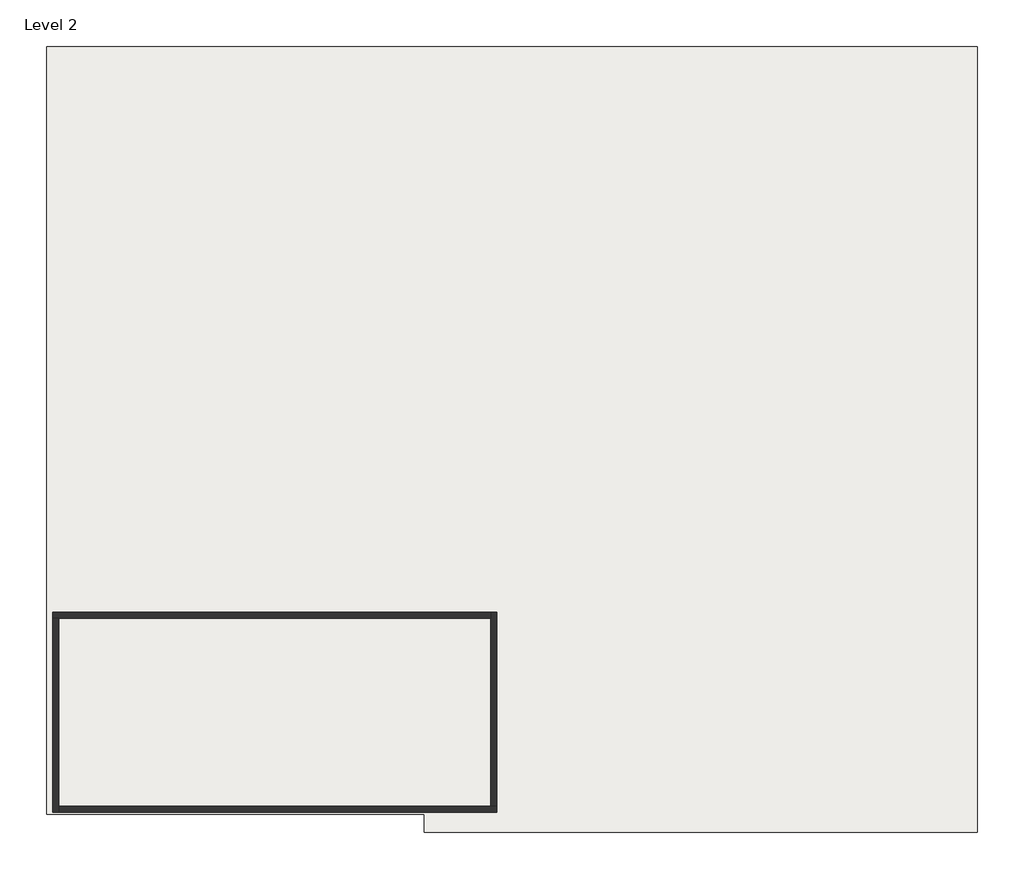
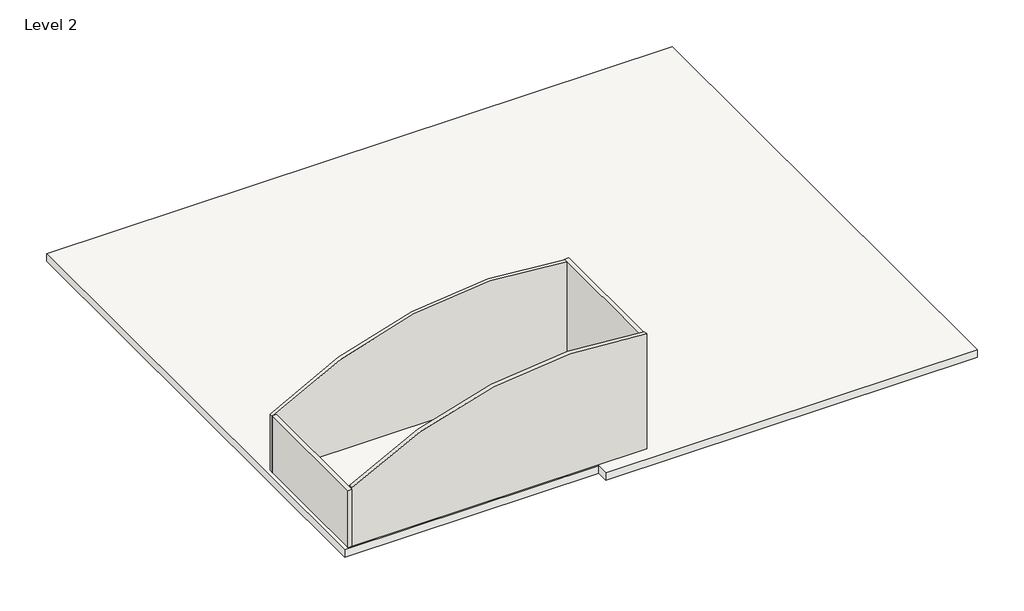
# One storey: 4 walls, 1 slab.
"""IFC4 building model written with IfcOpenShell, lengths in millimetres."""

from ifc_helpers import new_model, si_unit, frame, origin, place, context, project, spatial, polyline, circle_curve, outline, extrude, faceted_brep, element, save
from ifc_brep_helpers import plane_surface, cylinder_surface, advanced_brep

model = new_model("IFC4")

# Units and contexts
model_context = context("Model", 3, world=origin())
ifc_project = project(units=[si_unit("LENGTHUNIT", "METRE", prefix="MILLI")], contexts=[model_context])

# Site, building, storey
site = spatial("IfcSite", under=ifc_project)
building = spatial("IfcBuilding", under=site)
storey = spatial("IfcBuildingStorey", under=building, Name="Level 2", Elevation=5696.0)

# Slab
placement = place(None, origin())
element("IfcSlab", 1, ObjectType="Generic 5\"", at=placement, inside=storey, context=model_context, shape_type="SweptSolid", body=[
    extrude(outline(polyline([(-21609.2828737, 17887.7099289), (9680.512328, 17887.7099289), (9680.512328, -8525.0900711), (-8912.287672, -8525.0900711), (-8912.287672, -7915.4900711), (-21609.2828737, -7915.4900711), (-21609.2828737, 17887.7099289)])), frame((0.0, 0.0, 5296.0), z_axis=(0.0, 0.0, 1.0), x_axis=(1.0, 0.0, 0.0)), (0.0, 0.0, 1.0), 400.0),
])

# Walls
element("IfcWall", 2, ObjectType="Generic - 9\"", at=placement, inside=storey, context=model_context, shape_type="AdvancedBrep", body=[
    advanced_brep(
    [(-6474.0828737, -7653.4043927, 5696.0), (-6674.0828737, -7653.4043927, 5696.0), (-21204.4828737, -7653.4043927, 5696.0), (-21204.4828737, -7653.4043927, 8808.0736123), (-6474.0828737, -7653.4043927, 11775.1398494), (-6474.0828737, -7653.4043927, 11709.4744332), (-6474.0828737, -7853.4043927, 5696.0), (-6474.0828737, -7853.4043927, 11775.1398494), (-21204.4828737, -7853.4043927, 8808.0736123), (-21204.4828737, -7853.4043927, 8723.1502964), (-21204.4828737, -7853.4043927, 5696.0)],
    [
        (0, 1),
        (1, 2),
        (2, 3),
        (3, 4, circle_curve(frame((-9994.1657461, -7653.4043927, -8797.995189), z_axis=(0.0, 1.0, 0.0), x_axis=(1.0, 0.0, 0.0)), 20872.107434)),
        (4, 5),
        (5, 0),
        (6, 7),
        (7, 8, circle_curve(frame((-9994.1657461, -7853.4043927, -8797.995189), z_axis=(0.0, -1.0, 0.0), x_axis=(1.0, 0.0, 0.0)), 20872.107434)),
        (8, 9),
        (9, 10),
        (10, 6),
        (4, 7),
        (6, 0),
        (2, 10),
        (8, 3),
    ],
    [
        plane_surface(frame((-6574.0828737, -7653.4043927, 5696.0), z_axis=(0.0, 1.0, 0.0), x_axis=(-1.0, 0.0, 0.0))),
        plane_surface(frame((-6574.0828737, -7853.4043927, 5696.0), z_axis=(0.0, -1.0, 0.0), x_axis=(1.0, 0.0, 0.0))),
        plane_surface(frame((-6474.0828737, -1657.4043927, 5696.0), z_axis=(1.0, 0.0, 0.0), x_axis=(0.0, 1.0, 0.0))),
        plane_surface(frame((-21204.4828737, -7753.4043927, 5696.0), z_axis=(-1.0, 0.0, 0.0), x_axis=(0.0, 1.0, 0.0))),
        plane_surface(frame((-6574.0828737, -7653.4043927, 5696.0), z_axis=(0.0, 0.0, -1.0), x_axis=(0.0, -1.0, 0.0))),
        cylinder_surface(frame((-9994.1657461, -7853.4043927, -8797.995189), z_axis=(0.0, 1.0, 0.0), x_axis=(1.0, 0.0, 0.0)), 20872.107434),
    ],
    [
        (0, [[1, 2, 3, 4, 5, 6]]),
        (1, [[7, 8, 9, 10, 11]]),
        (2, [[-6, -5, 12, -7, 13]]),
        (3, [[-3, 14, -10, -9, 15]]),
        (4, [[-2, -1, -13, -11, -14]]),
        (5, [[-4, -15, -8, -12]]),
    ],
),
])
element("IfcWall", 3, ObjectType="Generic - 9\"", at=placement, inside=storey, context=model_context, shape_type="Brep", body=[
    faceted_brep([(-6674.0828737, -1123.0109022, 5696.0), (-6674.0828737, -1323.0109022, 5696.0), (-6674.0828737, -7653.4043927, 5696.0), (-6674.0828737, -7653.4043927, 11709.4744332), (-6674.0828737, -1123.0109022, 11709.4744332), (-6674.0828737, -1123.0109022, 11691.648024), (-6474.0828737, -1123.0109022, 5696.0), (-6474.0828737, -1123.0109022, 11709.4744332), (-6474.0828737, -7653.4043927, 11709.4744332), (-6474.0828737, -7653.4043927, 5696.0)], [[[0, 1, 2, 3, 4, 5]], [[6, 7, 8, 9]], [[2, 1, 0, 6, 9]], [[4, 3, 8, 7]], [[3, 2, 9, 8]], [[0, 5, 4, 7, 6]]]),
])
element("IfcWall", 4, ObjectType="Generic - 9\"", at=placement, inside=storey, context=model_context, shape_type="AdvancedBrep", body=[
    advanced_brep(
    [(-21404.4828737, -1323.0109022, 5696.0), (-21204.4828737, -1323.0109022, 5696.0), (-6674.0828737, -1323.0109022, 5696.0), (-6674.0828737, -1323.0109022, 11691.648024), (-21404.4828737, -1323.0109022, 8677.877941), (-21404.4828737, -1123.0109022, 5696.0), (-21404.4828737, -1123.0109022, 8677.877941), (-6674.0828737, -1123.0109022, 11691.648024), (-6674.0828737, -1123.0109022, 5696.0)],
    [
        (0, 1),
        (1, 2),
        (2, 3),
        (3, 4, circle_curve(frame((-10324.9947486, -1323.0109022, -7969.5581139), z_axis=(0.0, -1.0, 0.0), x_axis=(-1.0, 0.0, 0.0)), 19997.3044262)),
        (4, 0),
        (5, 6),
        (6, 7, circle_curve(frame((-10324.9947486, -1123.0109022, -7969.5581139), z_axis=(0.0, 1.0, 0.0), x_axis=(-1.0, 0.0, 0.0)), 19997.3044262)),
        (7, 8),
        (8, 5),
        (2, 8),
        (7, 3),
        (4, 6),
        (5, 0),
    ],
    [
        plane_surface(frame((-21204.4828737, -1323.0109022, 5696.0), z_axis=(0.0, -1.0, 0.0), x_axis=(1.0, 0.0, 0.0))),
        plane_surface(frame((-21204.4828737, -1123.0109022, 5696.0), z_axis=(0.0, 1.0, 0.0), x_axis=(-1.0, 0.0, 0.0))),
        plane_surface(frame((-6674.0828737, -1657.4043927, 5696.0), z_axis=(1.0, 0.0, 0.0), x_axis=(0.0, -1.0, 0.0))),
        plane_surface(frame((-21404.4828737, -7753.4043927, 5696.0), z_axis=(-1.0, 0.0, 0.0), x_axis=(0.0, -1.0, 0.0))),
        plane_surface(frame((-21304.4828737, -1323.0109022, 5696.0), z_axis=(0.0, 0.0, -1.0), x_axis=(0.0, 1.0, 0.0))),
        cylinder_surface(frame((-10324.9947486, -1123.0109022, -7969.5581139), z_axis=(0.0, -1.0, 0.0), x_axis=(-1.0, 0.0, 0.0)), 19997.3044262),
    ],
    [
        (0, [[1, 2, 3, 4, 5]]),
        (1, [[6, 7, 8, 9]]),
        (2, [[-3, 10, -8, 11]]),
        (3, [[-5, 12, -6, 13]]),
        (4, [[-2, -1, -13, -9, -10]]),
        (5, [[-4, -11, -7, -12]]),
    ],
),
])
element("IfcWall", 5, ObjectType="Generic - 9\"", at=placement, inside=storey, context=model_context, shape_type="Brep", body=[
    faceted_brep([(-21204.4828737, -7853.4043927, 5696.0), (-21204.4828737, -7653.4043927, 5696.0), (-21204.4828737, -1323.0109022, 5696.0), (-21204.4828737, -1323.0109022, 8723.1502964), (-21204.4828737, -7853.4043927, 8723.1502964), (-21404.4828737, -7853.4043927, 5696.0), (-21404.4828737, -7853.4043927, 8723.1502964), (-21404.4828737, -1323.0109022, 8723.1502964), (-21404.4828737, -1323.0109022, 8677.877941), (-21404.4828737, -1323.0109022, 5696.0)], [[[0, 1, 2, 3, 4]], [[5, 6, 7, 8, 9]], [[2, 1, 0, 5, 9]], [[4, 3, 7, 6]], [[0, 4, 6, 5]], [[3, 2, 9, 8, 7]]]),
])

save(model, "model.ifc")

# Revit data of these elements
# Type "Generic 5\""
#   Function = 0
#   Layers, outside or top first: 1' - 3.74803" no material (function 1)
# Type "Generic - 9\""
#   Layers, outside or top first: 0' - 7.87402" no material (function 1)
# Element 1 (IfcSlab, "Generic 5\"")
#   built-in parameter 1001955 = 3.14159 (stored number, unit not read)
#   Height Offset From Level = 0' - 0"
#   Phase Created = New Construction
#   Materials on its faces: "Default Roof"
# Element 2 (IfcWall, "Generic - 9\"")
#   Top Offset = 0' - 0"
#   Base Offset = 0' - 0"
#   Unconnected Height = 20' - 0"
#   wall height = 20' - 0"
#   Phase Created = New Construction
#   Base Constraint = Level 2
#   Materials on its faces: "Default Wall"
# Element 3 (IfcWall, "Generic - 9\"")
#   Top Offset = 0' - 0"
#   Base Offset = 0' - 0"
#   Unconnected Height = 19' - 8.75096"
#   wall height = 19' - 8.75096"
#   Phase Created = New Construction
#   Base Constraint = Level 2
#   Materials on its faces: "Default Wall"
# Element 4 (IfcWall, "Generic - 9\"")
#   Top Offset = 0' - 0"
#   Base Offset = 0' - 0"
#   Unconnected Height = 19' - 7.3077"
#   wall height = 19' - 7.3077"
#   Phase Created = New Construction
#   Base Constraint = Level 2
#   Materials on its faces: "Default Wall"
# Element 5 (IfcWall, "Generic - 9\"")
#   Top Offset = 0' - 0"
#   Base Offset = 0' - 0"
#   Unconnected Height = 9' - 11.17915"
#   wall height = 9' - 11.17915"
#   Phase Created = New Construction
#   Base Constraint = Level 2
#   Materials on its faces: "Default Wall"
# Materials
#   "Default Roof": colour RGB 80 80 80, transparency 0
#   "Default Wall": colour RGB 80 80 80, transparency 0
